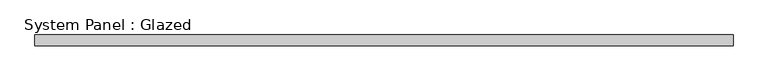
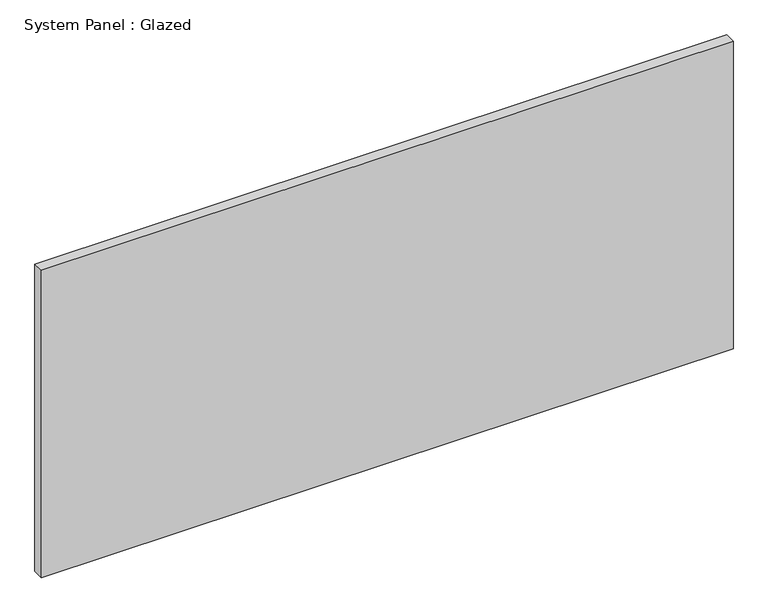
"""IFC4 building model written with IfcOpenShell, lengths in millimetres: plate geometry, System Panel : Glazed."""

from ifc_helpers import new_model, si_unit, origin, origin_with_axes, place, context, project, spatial, polyline, outline, extrude, source, transform, mapped, element, save


def system_panel_glazed_4dc74c46(model_context):
    return source(origin(), model_context, "Body", "SweptSolid", [
        extrude(outline(polyline([(806.45, 19.05), (-806.45, 19.05), (-806.45, 44.45), (806.45, 44.45), (806.45, 19.05)])), origin_with_axes(), (0.0, 0.0, 1.0), 757.5270145),
    ])


if __name__ == "__main__":
    model = new_model("IFC4")
    model_context = context("Model", 3, world=origin())
    ifc_project = project(units=[si_unit("LENGTHUNIT", "METRE", prefix="MILLI")], contexts=[model_context])
    site = spatial("IfcSite", under=ifc_project)
    building = spatial("IfcBuilding", under=site)
    placement = place(None, origin())
    system_panel_glazed_shape = system_panel_glazed_4dc74c46(model_context)
    element("IfcPlate", 1, ObjectType="System Panel : Glazed", at=placement, inside=building, context=model_context, shape_type="MappedRepresentation", body=[
        mapped(system_panel_glazed_shape, transform((0.0, 0.0, 0.0), x_axis=(1.0, 0.0, 0.0), y_axis=(0.0, 1.0, 0.0), z_axis=(0.0, 0.0, 1.0))),
    ])
    save(model, "model.ifc")

# Revit data of these elements
# Type "System Panel : Glazed"
#   Construction Type Id = "GSP4R"
#   Analytic Construction = "1/8 in Pilkington single glazing"
#   Visual Light Transmittance = 0.9
#   Solar Heat Gain Coefficient = 0.86
#   Heat Transfer Coefficient (U) = 1.18115 BTU/(h·ft²·°F)
#   Define Thermal Properties by = 1
# Element 1 (IfcPlate, "System Panel : Glazed")
#   Materials on its faces: "Glass"
# Materials
#   "Glass": class "Glass", colour RGB 0 128 192, transparency 0.75, Description = "Soda Lime Glass", Cost = 0
